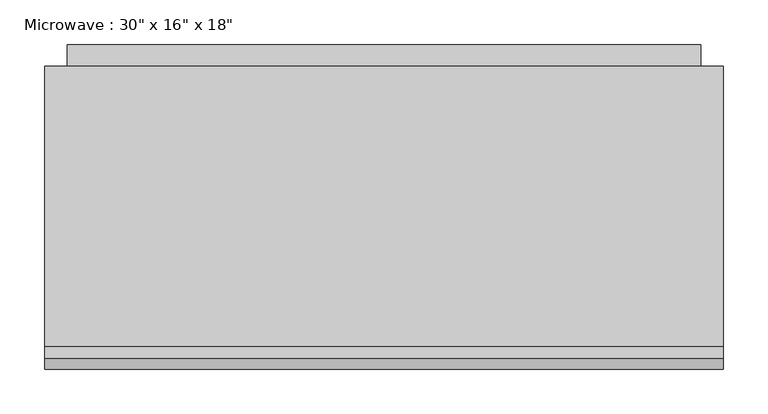
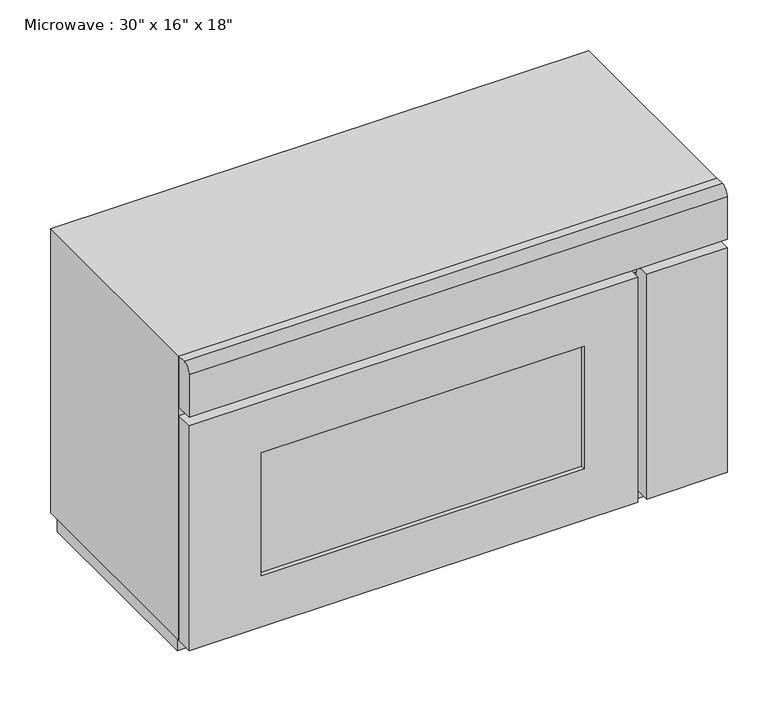
"""IFC4 building model written with IfcOpenShell, lengths in millimetres: proxy geometry."""

from ifc_helpers import new_model, si_unit, point, frame, frame_2d, origin, place, context, project, spatial, polyline, circle_curve, trimmed, segment, composite_curve, outline, extrude, source, transform, mapped, element, save


def proxy_487063f8(model_context):
    return source(origin(), model_context, "Body", "SweptSolid", [
        extrude(outline(polyline([(678.4897523, -529.5906621), (220.8928773, -529.5906621), (220.8928773, -523.2406621), (678.4897523, -523.2406621), (678.4897523, -529.5906621)])), frame((0.0, 0.0, 1022.35), z_axis=(0.0, 0.0, 1.0), x_axis=(1.0, 0.0, 0.0)), (0.0, 0.0, 1.0), 184.15),
        extrude(outline(polyline([(1282.7, 754.6897523), (1282.7, 119.2928773), (946.15, 119.2928773), (946.15, 754.6897523), (1282.7, 754.6897523)]), holes=[polyline([(1206.5, 678.4897523), (1022.35, 678.4897523), (1022.35, 220.8928773), (1206.5, 220.8928773), (1206.5, 678.4897523)])]), frame((0.0, -535.9406621, 0.0), z_axis=(0.0, 1.0, 0.0), x_axis=(0.0, 0.0, 1.0)), (0.0, 0.0, 1.0), 25.4),
        extrude(outline(polyline([(881.2928773, -535.9406621), (767.3897523, -535.9406621), (767.3897523, -510.5406621), (881.2928773, -510.5406621), (881.2928773, -535.9406621)])), frame((0.0, 0.0, 946.15), z_axis=(0.0, 0.0, 1.0), x_axis=(1.0, 0.0, 0.0)), (0.0, 0.0, 1.0), 336.55),
        extrude(outline(composite_curve([segment(polyline([(-523.2406621, 1371.6), (-510.5406621, 1371.6), (-510.5406621, 1295.4), (-535.9406621, 1295.4), (-535.9406621, 1358.9)]), True, "CONTINUOUS"), segment(trimmed(circle_curve(frame_2d((-523.2406621, 1358.9)), 12.7), [point((-535.9406621, 1358.9))], [point((-523.2406621, 1371.6))], False, "CARTESIAN"), True, "CONTINUOUS")], self_intersect=False)), frame((119.2928773, 0.0, 0.0), z_axis=(1.0, 0.0, 0.0), x_axis=(0.0, 1.0, 0.0)), (0.0, 0.0, 1.0), 762.0),
        extrude(outline(polyline([(-171.3839932, 1346.2), (-171.3839932, 961.946551), (-196.7839932, 936.546551), (-196.7839932, 1346.2), (-171.3839932, 1346.2)])), frame((144.6928773, 0.0, 0.0), z_axis=(1.0, 0.0, 0.0), x_axis=(0.0, 1.0, 0.0)), (0.0, 0.0, 1.0), 711.2),
        extrude(outline(polyline([(1371.6, 881.2928773), (1371.6, 119.2928773), (946.15, 119.2928773), (946.15, 881.2928773), (1371.6, 881.2928773)]), holes=[polyline([(1271.0014904, 824.5397523), (1020.1764904, 824.5397523), (1020.1764904, 176.0460023), (1271.0014904, 176.0460023), (1271.0014904, 824.5397523)])]), frame((0.0, -510.5406621, 0.0), z_axis=(0.0, 1.0, 0.0), x_axis=(0.0, 0.0, 1.0)), (0.0, 0.0, 1.0), 314.9203125),
        extrude(outline(polyline([(871.7678773, -195.6203496), (871.7678773, -489.9031621), (128.8178773, -489.9031621), (128.8178773, -195.6203496), (871.7678773, -195.6203496)])), frame((0.0, 0.0, 914.4), z_axis=(0.0, 0.0, 1.0), x_axis=(1.0, 0.0, 0.0)), (0.0, 0.0, 1.0), 31.75),
    ])


if __name__ == "__main__":
    model = new_model("IFC4")
    model_context = context("Model", 3, world=origin())
    ifc_project = project(units=[si_unit("LENGTHUNIT", "METRE", prefix="MILLI")], contexts=[model_context])
    site = spatial("IfcSite", under=ifc_project)
    building = spatial("IfcBuilding", under=site)
    placement = place(None, origin())
    proxy_shape = proxy_487063f8(model_context)
    element("IfcBuildingElementProxy", 1, Name="Microwave : 30\" x 16\" x 18\"", ObjectType="Microwave : 30\" x 16\" x 18\"", at=placement, inside=building, context=model_context, shape_type="MappedRepresentation", body=[
        mapped(proxy_shape, transform((0.0, 0.0, 0.0), x_axis=(1.0, 0.0, 0.0), y_axis=(0.0, 1.0, 0.0), z_axis=(0.0, 0.0, 1.0))),
    ])
    save(model, "model.ifc")

# Revit data of these elements
# Type "Microwave : 30\" x 16\" x 18\""
#   Assembly Code = "E1090400"
#   Depth = 1' - 2 51/128"
#   Height = 1' - 6"
#   Width = 2' - 6"
#   Microwave Material = Laminate, Ivory, Matte
#   Default Elevation = 0
# Element 1 (IfcBuildingElementProxy, "Microwave : 30\" x 16\" x 18\"")
#   Materials on its faces: "Laminate, Ivory, Matte", "Glass"
# Materials
#   "Laminate, Ivory, Matte": class "Plastic", colour RGB 247 247 239, transparency 0, Description = "Plastic Laminate - Ivory, Matte", Cost = 0
#   "Glass": class "Glass", colour RGB 0 128 192, transparency 0.75, Description = "Soda Lime Glass", Cost = 0
